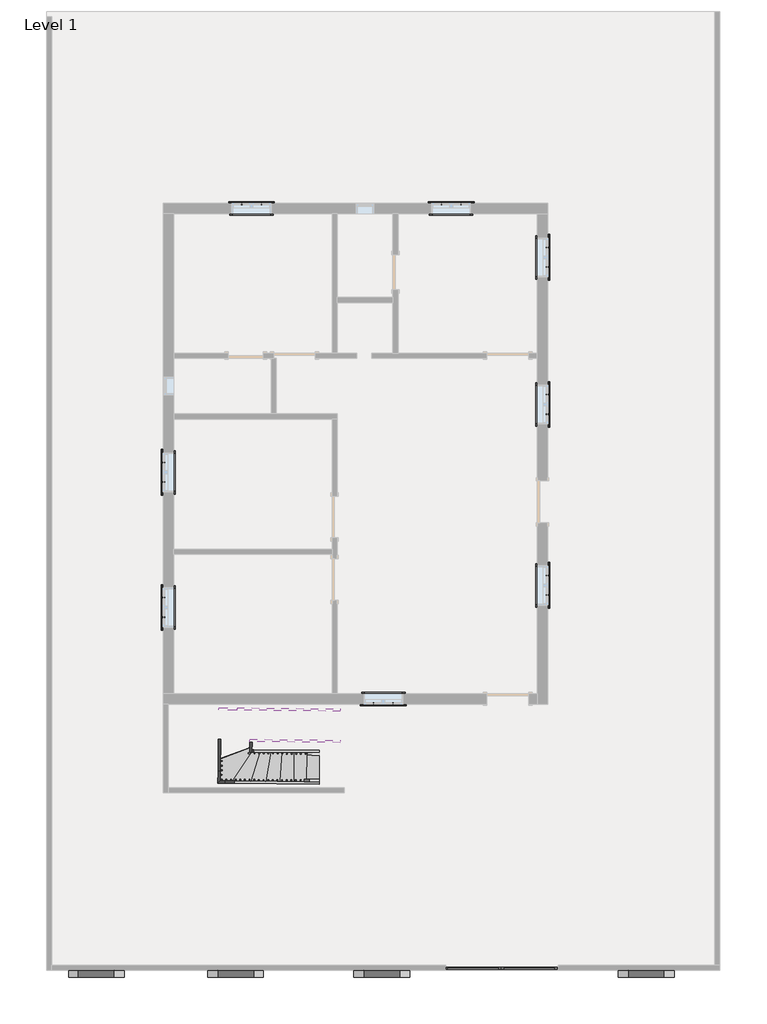
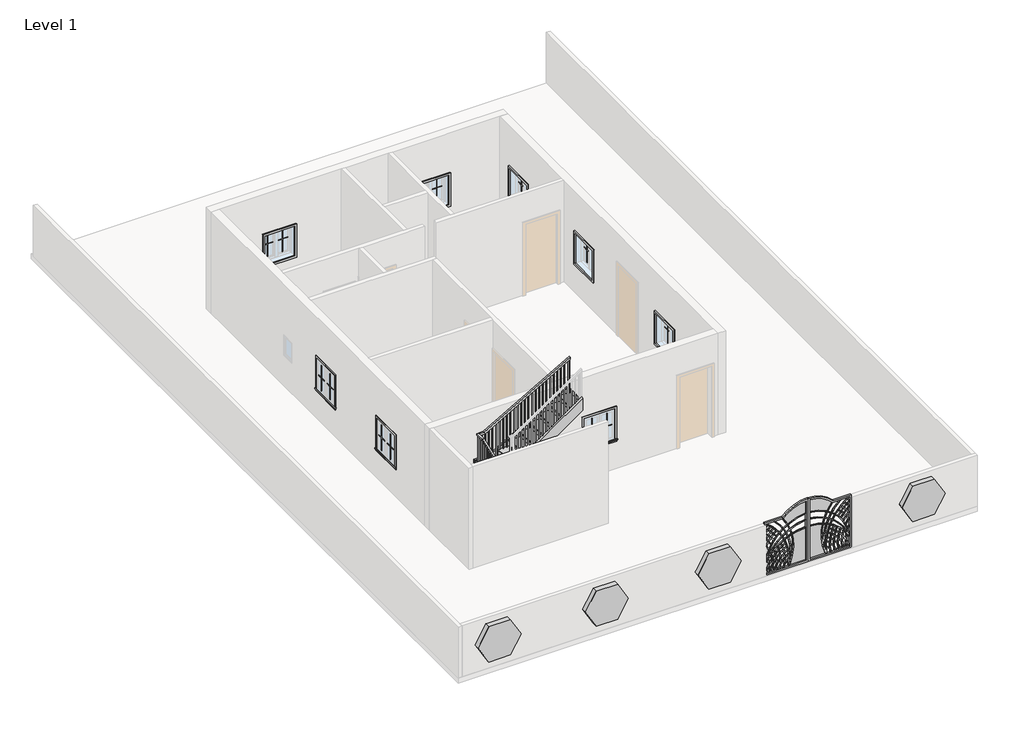
# One storey, part 2 of 2: 34 proxies, 9 members, 1 railing, 1 stair flight.
"""IFC4 building model written with IfcOpenShell, lengths in millimetres."""

from ifc_helpers import new_model, si_unit, frame, origin, place, context, project, spatial, polyline, outline, extrude, faceted_brep, transform, mapped, element, save
from components import generic_models_6bc30956, generic_models_1_generic_models_1_46fdab30, muntin_pattern_2x2_muntin_pattern_2x2_b3fe6957, muntin_pattern_2x2_muntin_pattern_2x2_3e0ecaf2, trim_window_exterior_flat_with_sill_41619996, trim_window_interior_flat_picture_frame_51c85655, stair_flight_bcee568d

model = new_model("IFC4")

# Units and contexts
model_context = context("Model", 3, world=origin())
ifc_project = project(units=[si_unit("LENGTHUNIT", "METRE", prefix="MILLI")], contexts=[model_context])

# Site, building, storey
site = spatial("IfcSite", under=ifc_project)
building = spatial("IfcBuilding", under=site)
storey = spatial("IfcBuildingStorey", under=building, Name="Level 1", Elevation=0.0)

# Proxies
placement = place(None, origin())
generic_models_shape = generic_models_6bc30956(model_context)
element("IfcBuildingElementProxy", 1, Name="Generic Models", at=placement, inside=storey, context=model_context, shape_type="MappedRepresentation", body=[
    mapped(generic_models_shape, transform((2009.5752168, -9655.81366, 0.0), x_axis=(1.0, 0.0, 0.0), y_axis=(0.0, 1.0, 0.0), z_axis=(0.0, 0.0, 1.0))),
])
generic_models_1_generic_models_1_shape = generic_models_1_generic_models_1_46fdab30(model_context)
element("IfcBuildingElementProxy", 2, Name="Generic Models 1 : Generic Models 1", ObjectType="Generic Models 1 : Generic Models 1", at=placement, inside=storey, context=model_context, shape_type="MappedRepresentation", body=[
    mapped(generic_models_1_generic_models_1_shape, transform((0.0, 0.0, 0.0), x_axis=(1.0, 0.0, 0.0), y_axis=(0.0, 1.0, 0.0), z_axis=(0.0, 0.0, 1.0))),
])
muntin_pattern_2x2_muntin_pattern_2x2_shape = muntin_pattern_2x2_muntin_pattern_2x2_b3fe6957(model_context)
element("IfcBuildingElementProxy", 3, Name="Muntin Pattern_2x2 : Muntin Pattern_2x2", ObjectType="Muntin Pattern_2x2 : Muntin Pattern_2x2", at=placement, inside=storey, context=model_context, shape_type="MappedRepresentation", body=[
    mapped(muntin_pattern_2x2_muntin_pattern_2x2_shape, transform((-3662.5622832, 7052.6782079, 984.25), x_axis=(1.0, 0.0, 0.0), y_axis=(0.0, 1.0, 0.0), z_axis=(0.0, 0.0, 1.0))),
])
element("IfcBuildingElementProxy", 4, Name="Muntin Pattern_2x2 : Muntin Pattern_2x2", ObjectType="Muntin Pattern_2x2 : Muntin Pattern_2x2", at=placement, inside=storey, context=model_context, shape_type="MappedRepresentation", body=[
    mapped(muntin_pattern_2x2_muntin_pattern_2x2_shape, transform((709.4127168, 7052.6782079, 984.25), x_axis=(1.0, 0.0, 0.0), y_axis=(0.0, 1.0, 0.0), z_axis=(0.0, 0.0, 1.0))),
])
element("IfcBuildingElementProxy", 5, Name="Muntin Pattern_2x2 : Muntin Pattern_2x2", ObjectType="Muntin Pattern_2x2 : Muntin Pattern_2x2", at=placement, inside=storey, context=model_context, shape_type="MappedRepresentation", body=[
    mapped(muntin_pattern_2x2_muntin_pattern_2x2_shape, transform((3028.7502168, 6095.4157079, 984.25), x_axis=(0.0, -1.0, 0.0), y_axis=(1.0, 0.0, 0.0), z_axis=(0.0, 0.0, 1.0))),
])
element("IfcBuildingElementProxy", 6, Name="Muntin Pattern_2x2 : Muntin Pattern_2x2", ObjectType="Muntin Pattern_2x2 : Muntin Pattern_2x2", at=placement, inside=storey, context=model_context, shape_type="MappedRepresentation", body=[
    mapped(muntin_pattern_2x2_muntin_pattern_2x2_shape, transform((3028.7502168, 2875.9657079, 984.25), x_axis=(0.0, -1.0, 0.0), y_axis=(1.0, 0.0, 0.0), z_axis=(0.0, 0.0, 1.0))),
])
element("IfcBuildingElementProxy", 7, Name="Muntin Pattern_2x2 : Muntin Pattern_2x2", ObjectType="Muntin Pattern_2x2 : Muntin Pattern_2x2", at=placement, inside=storey, context=model_context, shape_type="MappedRepresentation", body=[
    mapped(muntin_pattern_2x2_muntin_pattern_2x2_shape, transform((3028.7502168, -1086.4342921, 984.25), x_axis=(0.0, -1.0, 0.0), y_axis=(1.0, 0.0, 0.0), z_axis=(0.0, 0.0, 1.0))),
])
element("IfcBuildingElementProxy", 8, Name="Muntin Pattern_2x2 : Muntin Pattern_2x2", ObjectType="Muntin Pattern_2x2 : Muntin Pattern_2x2", at=placement, inside=storey, context=model_context, shape_type="MappedRepresentation", body=[
    mapped(muntin_pattern_2x2_muntin_pattern_2x2_shape, transform((-5372.2997832, 961.4407079, 984.25), x_axis=(0.0, 1.0, 0.0), y_axis=(-1.0, 0.0, 0.0), z_axis=(0.0, 0.0, 1.0))),
])
element("IfcBuildingElementProxy", 9, Name="Muntin Pattern_2x2 : Muntin Pattern_2x2", ObjectType="Muntin Pattern_2x2 : Muntin Pattern_2x2", at=placement, inside=storey, context=model_context, shape_type="MappedRepresentation", body=[
    mapped(muntin_pattern_2x2_muntin_pattern_2x2_shape, transform((-5372.2997832, -1997.6592921, 984.25), x_axis=(0.0, 1.0, 0.0), y_axis=(-1.0, 0.0, 0.0), z_axis=(0.0, 0.0, 1.0))),
])
element("IfcBuildingElementProxy", 10, Name="Muntin Pattern_2x2 : Muntin Pattern_2x2", ObjectType="Muntin Pattern_2x2 : Muntin Pattern_2x2", at=placement, inside=storey, context=model_context, shape_type="MappedRepresentation", body=[
    mapped(muntin_pattern_2x2_muntin_pattern_2x2_shape, transform((-347.8622832, -3888.3717921, 984.25), x_axis=(-1.0, 0.0, 0.0), y_axis=(0.0, -1.0, 0.0), z_axis=(0.0, 0.0, 1.0))),
])
muntin_pattern_2x2_muntin_pattern_2x2_2_shape = muntin_pattern_2x2_muntin_pattern_2x2_3e0ecaf2(model_context)
element("IfcBuildingElementProxy", 11, Name="Muntin Pattern_2x2 : Muntin Pattern_2x2", ObjectType="Muntin Pattern_2x2 : Muntin Pattern_2x2", at=placement, inside=storey, context=model_context, shape_type="MappedRepresentation", body=[
    mapped(muntin_pattern_2x2_muntin_pattern_2x2_2_shape, transform((-3233.9372832, 7052.6782079, 984.25), x_axis=(-1.0, 0.0, 0.0), y_axis=(0.0, -1.0, 0.0), z_axis=(0.0, 0.0, 1.0))),
])
element("IfcBuildingElementProxy", 12, Name="Muntin Pattern_2x2 : Muntin Pattern_2x2", ObjectType="Muntin Pattern_2x2 : Muntin Pattern_2x2", at=placement, inside=storey, context=model_context, shape_type="MappedRepresentation", body=[
    mapped(muntin_pattern_2x2_muntin_pattern_2x2_2_shape, transform((1138.0377168, 7052.6782079, 984.25), x_axis=(-1.0, 0.0, 0.0), y_axis=(0.0, -1.0, 0.0), z_axis=(0.0, 0.0, 1.0))),
])
element("IfcBuildingElementProxy", 13, Name="Muntin Pattern_2x2 : Muntin Pattern_2x2", ObjectType="Muntin Pattern_2x2 : Muntin Pattern_2x2", at=placement, inside=storey, context=model_context, shape_type="MappedRepresentation", body=[
    mapped(muntin_pattern_2x2_muntin_pattern_2x2_2_shape, transform((3028.7502168, 5666.7907079, 984.25), x_axis=(0.0, 1.0, 0.0), y_axis=(-1.0, 0.0, 0.0), z_axis=(0.0, 0.0, 1.0))),
])
element("IfcBuildingElementProxy", 14, Name="Muntin Pattern_2x2 : Muntin Pattern_2x2", ObjectType="Muntin Pattern_2x2 : Muntin Pattern_2x2", at=placement, inside=storey, context=model_context, shape_type="MappedRepresentation", body=[
    mapped(muntin_pattern_2x2_muntin_pattern_2x2_2_shape, transform((3028.7502168, 2447.3407079, 984.25), x_axis=(0.0, 1.0, 0.0), y_axis=(-1.0, 0.0, 0.0), z_axis=(0.0, 0.0, 1.0))),
])
element("IfcBuildingElementProxy", 15, Name="Muntin Pattern_2x2 : Muntin Pattern_2x2", ObjectType="Muntin Pattern_2x2 : Muntin Pattern_2x2", at=placement, inside=storey, context=model_context, shape_type="MappedRepresentation", body=[
    mapped(muntin_pattern_2x2_muntin_pattern_2x2_2_shape, transform((3028.7502168, -1515.0592921, 984.25), x_axis=(0.0, 1.0, 0.0), y_axis=(-1.0, 0.0, 0.0), z_axis=(0.0, 0.0, 1.0))),
])
element("IfcBuildingElementProxy", 16, Name="Muntin Pattern_2x2 : Muntin Pattern_2x2", ObjectType="Muntin Pattern_2x2 : Muntin Pattern_2x2", at=placement, inside=storey, context=model_context, shape_type="MappedRepresentation", body=[
    mapped(muntin_pattern_2x2_muntin_pattern_2x2_2_shape, transform((-5372.2997832, 1390.0657079, 984.25), x_axis=(0.0, -1.0, 0.0), y_axis=(1.0, 0.0, 0.0), z_axis=(0.0, 0.0, 1.0))),
])
element("IfcBuildingElementProxy", 17, Name="Muntin Pattern_2x2 : Muntin Pattern_2x2", ObjectType="Muntin Pattern_2x2 : Muntin Pattern_2x2", at=placement, inside=storey, context=model_context, shape_type="MappedRepresentation", body=[
    mapped(muntin_pattern_2x2_muntin_pattern_2x2_2_shape, transform((-5372.2997832, -1569.0342921, 984.25), x_axis=(0.0, -1.0, 0.0), y_axis=(1.0, 0.0, 0.0), z_axis=(0.0, 0.0, 1.0))),
])
element("IfcBuildingElementProxy", 18, Name="Muntin Pattern_2x2 : Muntin Pattern_2x2", ObjectType="Muntin Pattern_2x2 : Muntin Pattern_2x2", at=placement, inside=storey, context=model_context, shape_type="MappedRepresentation", body=[
    mapped(muntin_pattern_2x2_muntin_pattern_2x2_2_shape, transform((-776.4872832, -3888.3717921, 984.25), x_axis=(1.0, 0.0, 0.0), y_axis=(0.0, 1.0, 0.0), z_axis=(0.0, 0.0, 1.0))),
])
trim_window_exterior_flat_with_sill_shape = trim_window_exterior_flat_with_sill_41619996(model_context)
element("IfcBuildingElementProxy", 19, Name="Trim-Window-Exterior-Flat : with Sill", ObjectType="Trim-Window-Exterior-Flat : with Sill", at=placement, inside=storey, context=model_context, shape_type="MappedRepresentation", body=[
    mapped(trim_window_exterior_flat_with_sill_shape, transform((-3448.2497832, 7062.2032079, 1828.8), x_axis=(-1.0, 0.0, 0.0), y_axis=(0.0, 0.0, 1.0), z_axis=(0.0, 1.0, 0.0))),
])
element("IfcBuildingElementProxy", 20, Name="Trim-Window-Exterior-Flat : with Sill", ObjectType="Trim-Window-Exterior-Flat : with Sill", at=placement, inside=storey, context=model_context, shape_type="MappedRepresentation", body=[
    mapped(trim_window_exterior_flat_with_sill_shape, transform((923.7252168, 7062.2032079, 1828.8), x_axis=(-1.0, 0.0, 0.0), y_axis=(0.0, 0.0, 1.0), z_axis=(0.0, 1.0, 0.0))),
])
element("IfcBuildingElementProxy", 21, Name="Trim-Window-Exterior-Flat : with Sill", ObjectType="Trim-Window-Exterior-Flat : with Sill", at=placement, inside=storey, context=model_context, shape_type="MappedRepresentation", body=[
    mapped(trim_window_exterior_flat_with_sill_shape, transform((3038.2752168, 5881.1032079, 1828.8), x_axis=(0.0, 1.0, 0.0), y_axis=(0.0, 0.0, 1.0), z_axis=(1.0, 0.0, 0.0))),
])
element("IfcBuildingElementProxy", 22, Name="Trim-Window-Exterior-Flat : with Sill", ObjectType="Trim-Window-Exterior-Flat : with Sill", at=placement, inside=storey, context=model_context, shape_type="MappedRepresentation", body=[
    mapped(trim_window_exterior_flat_with_sill_shape, transform((3038.2752168, 2661.6532079, 1828.8), x_axis=(0.0, 1.0, 0.0), y_axis=(0.0, 0.0, 1.0), z_axis=(1.0, 0.0, 0.0))),
])
element("IfcBuildingElementProxy", 23, Name="Trim-Window-Exterior-Flat : with Sill", ObjectType="Trim-Window-Exterior-Flat : with Sill", at=placement, inside=storey, context=model_context, shape_type="MappedRepresentation", body=[
    mapped(trim_window_exterior_flat_with_sill_shape, transform((3038.2752168, -1300.7467921, 1828.8), x_axis=(0.0, 1.0, 0.0), y_axis=(0.0, 0.0, 1.0), z_axis=(1.0, 0.0, 0.0))),
])
element("IfcBuildingElementProxy", 24, Name="Trim-Window-Exterior-Flat : with Sill", ObjectType="Trim-Window-Exterior-Flat : with Sill", at=placement, inside=storey, context=model_context, shape_type="MappedRepresentation", body=[
    mapped(trim_window_exterior_flat_with_sill_shape, transform((-5381.8247832, 1175.7532079, 1828.8), x_axis=(0.0, -1.0, 0.0), y_axis=(0.0, 0.0, 1.0), z_axis=(-1.0, 0.0, 0.0))),
])
element("IfcBuildingElementProxy", 25, Name="Trim-Window-Exterior-Flat : with Sill", ObjectType="Trim-Window-Exterior-Flat : with Sill", at=placement, inside=storey, context=model_context, shape_type="MappedRepresentation", body=[
    mapped(trim_window_exterior_flat_with_sill_shape, transform((-5381.8247832, -1783.3467921, 1828.8), x_axis=(0.0, -1.0, 0.0), y_axis=(0.0, 0.0, 1.0), z_axis=(-1.0, 0.0, 0.0))),
])
element("IfcBuildingElementProxy", 26, Name="Trim-Window-Exterior-Flat : with Sill", ObjectType="Trim-Window-Exterior-Flat : with Sill", at=placement, inside=storey, context=model_context, shape_type="MappedRepresentation", body=[
    mapped(trim_window_exterior_flat_with_sill_shape, transform((-562.1747832, -3897.8967921, 1828.8), x_axis=(1.0, 0.0, 0.0), y_axis=(0.0, 0.0, 1.0), z_axis=(0.0, -1.0, 0.0))),
])
trim_window_interior_flat_picture_frame_shape = trim_window_interior_flat_picture_frame_51c85655(model_context)
element("IfcBuildingElementProxy", 27, Name="Trim-Window-Interior-Flat : Picture Frame", ObjectType="Trim-Window-Interior-Flat : Picture Frame", at=placement, inside=storey, context=model_context, shape_type="MappedRepresentation", body=[
    mapped(trim_window_interior_flat_picture_frame_shape, transform((-3448.2497832, 6833.6032079, 1828.8), x_axis=(1.0, 0.0, 0.0), y_axis=(0.0, 0.0, 1.0), z_axis=(0.0, -1.0, 0.0))),
])
element("IfcBuildingElementProxy", 28, Name="Trim-Window-Interior-Flat : Picture Frame", ObjectType="Trim-Window-Interior-Flat : Picture Frame", at=placement, inside=storey, context=model_context, shape_type="MappedRepresentation", body=[
    mapped(trim_window_interior_flat_picture_frame_shape, transform((923.7252168, 6833.6032079, 1828.8), x_axis=(1.0, 0.0, 0.0), y_axis=(0.0, 0.0, 1.0), z_axis=(0.0, -1.0, 0.0))),
])
element("IfcBuildingElementProxy", 29, Name="Trim-Window-Interior-Flat : Picture Frame", ObjectType="Trim-Window-Interior-Flat : Picture Frame", at=placement, inside=storey, context=model_context, shape_type="MappedRepresentation", body=[
    mapped(trim_window_interior_flat_picture_frame_shape, transform((2809.6752168, 5881.1032079, 1828.8), x_axis=(0.0, -1.0, 0.0), y_axis=(0.0, 0.0, 1.0), z_axis=(-1.0, 0.0, 0.0))),
])
element("IfcBuildingElementProxy", 30, Name="Trim-Window-Interior-Flat : Picture Frame", ObjectType="Trim-Window-Interior-Flat : Picture Frame", at=placement, inside=storey, context=model_context, shape_type="MappedRepresentation", body=[
    mapped(trim_window_interior_flat_picture_frame_shape, transform((2809.6752168, 2661.6532079, 1828.8), x_axis=(0.0, -1.0, 0.0), y_axis=(0.0, 0.0, 1.0), z_axis=(-1.0, 0.0, 0.0))),
])
element("IfcBuildingElementProxy", 31, Name="Trim-Window-Interior-Flat : Picture Frame", ObjectType="Trim-Window-Interior-Flat : Picture Frame", at=placement, inside=storey, context=model_context, shape_type="MappedRepresentation", body=[
    mapped(trim_window_interior_flat_picture_frame_shape, transform((2809.6752168, -1300.7467921, 1828.8), x_axis=(0.0, -1.0, 0.0), y_axis=(0.0, 0.0, 1.0), z_axis=(-1.0, 0.0, 0.0))),
])
element("IfcBuildingElementProxy", 32, Name="Trim-Window-Interior-Flat : Picture Frame", ObjectType="Trim-Window-Interior-Flat : Picture Frame", at=placement, inside=storey, context=model_context, shape_type="MappedRepresentation", body=[
    mapped(trim_window_interior_flat_picture_frame_shape, transform((-5153.2247832, 1175.7532079, 1828.8), x_axis=(0.0, 1.0, 0.0), y_axis=(0.0, 0.0, 1.0), z_axis=(1.0, 0.0, 0.0))),
])
element("IfcBuildingElementProxy", 33, Name="Trim-Window-Interior-Flat : Picture Frame", ObjectType="Trim-Window-Interior-Flat : Picture Frame", at=placement, inside=storey, context=model_context, shape_type="MappedRepresentation", body=[
    mapped(trim_window_interior_flat_picture_frame_shape, transform((-5153.2247832, -1783.3467921, 1828.8), x_axis=(0.0, 1.0, 0.0), y_axis=(0.0, 0.0, 1.0), z_axis=(1.0, 0.0, 0.0))),
])
element("IfcBuildingElementProxy", 34, Name="Trim-Window-Interior-Flat : Picture Frame", ObjectType="Trim-Window-Interior-Flat : Picture Frame", at=placement, inside=storey, context=model_context, shape_type="MappedRepresentation", body=[
    mapped(trim_window_interior_flat_picture_frame_shape, transform((-562.1747832, -3669.2967921, 1828.8), x_axis=(-1.0, 0.0, 0.0), y_axis=(0.0, 0.0, 1.0), z_axis=(0.0, 1.0, 0.0))),
])

# Members
element("IfcMember", 35, ObjectType="Stringer - 2\" Width", at=placement, inside=storey, context=model_context, shape_type="SweptSolid", body=[
    extrude(outline(polyline([(-105.6395382, -202.4353776), (0.0, 0.0), (2328.2458671, 0.0), (2169.1880402, -304.8), (90.52017, -304.8), (-105.6395382, -202.4353776)])), frame((-1968.9977307, -5651.1672049, 228.3413982), z_axis=(0.010736031619565219, 0.9999423671517593, 0.0), x_axis=(-0.8864958884204133, 0.009517996437940355, 0.4626385711951713)), (0.0, 0.0, 1.0), 50.8),
])
element("IfcMember", 36, ObjectType="Stringer - 2\" Width", at=placement, inside=storey, context=model_context, shape_type="SweptSolid", body=[
    extrude(outline(polyline([(-4032.4327287, -5578.2098967), (-4032.9781191, -5629.006969), (-4182.4018504, -5627.4026586), (-4131.0593878, -5577.1509768), (-4032.4327287, -5578.2098967)])), frame((0.0, 0.0, 961.6719334), z_axis=(0.0, 0.0, 1.0), x_axis=(1.0, 0.0, 0.0)), (0.0, 0.0, 1.0), 343.8058061),
])
element("IfcMember", 37, ObjectType="Stringer - 2\" Width", at=placement, inside=storey, context=model_context, shape_type="SweptSolid", body=[
    extrude(outline(polyline([(-4131.0593878, -5577.1509768), (-4182.4018504, -5627.4026586), (-4179.6442274, -5370.5606366), (-4128.8471552, -5371.106027), (-4131.0593878, -5577.1509768)])), frame((0.0, 0.0, 961.6719334), z_axis=(0.0, 0.0, 1.0), x_axis=(1.0, 0.0, 0.0)), (0.0, 0.0, 1.0), 343.8058061),
])
element("IfcMember", 38, ObjectType="Stringer - 2\" Width", at=placement, inside=storey, context=model_context, shape_type="SweptSolid", body=[
    extrude(outline(polyline([(110.9788635, -325.4014815), (0.0, 0.0), (1419.3210826, 0.0), (1526.5904374, -314.5248191), (1494.6989405, -325.4014816), (110.9788635, -325.4014815)])), frame((-4128.8471552, -5371.106027, 961.6719334), z_axis=(-0.9999423671517594, 0.010736031619565323, 0.0), x_axis=(0.01016131936269789, 0.9464142894665318, 0.3227951986668468)), (0.0, 0.0, 1.0), 50.8),
])
element("IfcMember", 39, ObjectType="Stringer - 2\" Width", at=placement, inside=storey, context=model_context, shape_type="SweptSolid", body=[
    extrude(outline(polyline([(-4165.2220526, -4027.2948827), (-4164.6766622, -3976.4978105), (-3763.6581151, -3980.8034064), (-3764.2035055, -4031.6004787), (-4165.2220526, -4027.2948827)])), frame((0.0, 0.0, 1430.0968076), z_axis=(0.0, 0.0, 1.0), x_axis=(1.0, 0.0, 0.0)), (0.0, 0.0, 1.0), 322.0391291),
])
element("IfcMember", 40, ObjectType="Stringer - 2\" Width", at=placement, inside=storey, context=model_context, shape_type="SweptSolid", body=[
    extrude(outline(polyline([(-111.9640108, -160.4153284), (0.0, 0.0), (1801.1015507, 0.0), (1588.362339, -304.8), (94.9016984, -304.8), (-111.9640108, -160.4153284)])), frame((-1961.6349602, -4965.4067295, 195.6246848), z_axis=(0.010736031619565368, 0.9999423671517593, 0.0), x_axis=(-0.8199685195580251, 0.008803715336213087, 0.5723409137307062)), (0.0, 0.0, 1.0), 50.8),
])
element("IfcMember", 41, ObjectType="Stringer - 2\" Width", at=placement, inside=storey, context=model_context, shape_type="SweptSolid", body=[
    extrude(outline(polyline([(451.3522078, -304.8), (7.554265, -5.1014262), (10.999279, 0.0), (408.4725128, 0.0), (831.8908901, -285.9361695), (819.1520678, -304.8), (451.3522078, -304.8)])), frame((-3438.4815323, -4949.5503441, 881.1097108), z_axis=(-0.9999423671517593, 0.0107360316195659, 0.0), x_axis=(0.006008376943933793, 0.5596137266499716, 0.8287317879455516)), (0.0, 0.0, 1.0), 50.8),
])
element("IfcMember", 42, ObjectType="Stringer - 2\" Width", at=placement, inside=storey, context=model_context, shape_type="SweptSolid", body=[
    extrude(outline(polyline([(215.732707, -304.8), (0.0, 0.0), (2421.4097535, 0.0), (2637.1424605, -304.8), (215.732707, -304.8)])), frame((-3486.8243477, -4720.4181286, 1357.1256311), z_axis=(0.010736031619565212, 0.9999423671517593, 0.0), x_axis=(0.8161886957592972, -0.008763132689499912, 0.5777189804915567)), (0.0, 0.0, 1.0), 50.8),
])
element("IfcMember", 43, ObjectType="Stringer - 2\" Width", at=placement, inside=storey, context=model_context, shape_type="SweptSolid", body=[
    extrude(outline(polyline([(161.6856691, -278.5084291), (0.0, 0.0), (2614.6236412, 0.0), (2776.3093103, -278.508429), (161.6856691, -278.5084291)])), frame((-3764.2035055, -4031.6004787, 1430.0968076), z_axis=(0.010736031619565321, 0.9999423671517593, 0.0), x_axis=(0.8647780740833304, -0.009284819857879248, 0.5020683964410951)), (0.0, 0.0, 1.0), 50.8),
])

# Railing
element("IfcRailing", 44, ObjectType="Handrail - Rectangular", at=placement, inside=storey, context=model_context, shape_type="SolidModel", body=[
    faceted_brep([(-1968.4523403, -5600.3701326, 1083.7333333), (-1968.4523403, -5600.3701326, 1026.1388957), (-1967.9069499, -5549.5730604, 1026.1388957), (-1967.9069499, -5549.5730604, 1083.7333333), (-4009.5042766, -5578.4560715, 2174.1579081), (-4022.2220752, -5578.319525, 2123.3579081), (-4021.6766848, -5527.5224527, 2123.3579081), (-4008.9588862, -5527.6589993, 2174.1579081), (-4131.0593878, -5577.1509768, 2174.1579081), (-4131.0593878, -5577.1509768, 2123.3579081), (-4079.7169251, -5526.8992949, 2123.3579081), (-4079.7169251, -5526.8992949, 2174.1579081), (-4129.1695675, -5401.1351667, 2174.1579081), (-4129.079122, -5392.7111679, 2123.3579081), (-4078.2820498, -5393.2565584, 2123.3579081), (-4078.3724953, -5401.6805571, 2174.1579081), (-4117.5603361, -4319.8639155, 2542.9490097), (-4117.4698906, -4311.4399167, 2492.1490097), (-4066.6728183, -4311.9853071, 2492.1490097), (-4066.7632639, -4320.4093059, 2542.9490097), (-4114.4249804, -4027.8402731, 2542.9490097), (-4114.4249804, -4027.8402731, 2492.1490097), (-4064.1732985, -4079.1827358, 2492.1490097), (-4064.1732985, -4079.1827358, 2542.9490097), (-3933.3337165, -4029.7845867, 2542.9490097), (-3919.5861077, -4029.93219, 2492.1490097), (-3920.1314981, -4080.7292622, 2492.1490097), (-3933.8791069, -4080.581659, 2542.9490097), (-1503.1343086, -4055.8767882, 3962.4), (-1503.679699, -4106.6738604, 3962.4), (-1503.679699, -4106.6738604, 3903.5701828), (-1503.1343086, -4055.8767882, 3903.5701828)], [[[0, 1, 2, 3]], [[1, 0, 4, 5]], [[2, 1, 5, 6]], [[3, 2, 6, 7]], [[0, 3, 7, 4]], [[5, 4, 8, 9]], [[6, 5, 9, 10]], [[7, 6, 10, 11]], [[4, 7, 11, 8]], [[9, 8, 12, 13]], [[10, 9, 13, 14]], [[11, 10, 14, 15]], [[8, 11, 15, 12]], [[13, 12, 16, 17]], [[14, 13, 17, 18]], [[15, 14, 18, 19]], [[12, 15, 19, 16]], [[17, 16, 20, 21]], [[18, 17, 21, 22]], [[19, 18, 22, 23]], [[16, 19, 23, 20]], [[21, 20, 24, 25]], [[22, 21, 25, 26]], [[23, 22, 26, 27]], [[20, 23, 27, 24]], [[28, 29, 30, 31]], [[25, 24, 28, 31]], [[26, 25, 31, 30]], [[27, 26, 30, 29]], [[24, 27, 29, 28]]]),
    extrude(outline(polyline([(234.1631202, 19.05), (1226.6129544, 19.05), (1226.6129544, 0.0), (223.0368797, 0.0), (234.1631202, 19.05)])), frame((-1540.0233365, -4090.4077365, 4105.2796211), z_axis=(0.010736031619565153, 0.9999423671517594, 0.0), x_axis=(0.0, 0.0, -1.0)), (0.0, 0.0, 1.0), 19.05),
    extrude(outline(polyline([(234.1631202, 19.05), (1167.2730054, 19.05), (1167.2730054, 0.0), (223.0368798, 0.0), (234.1631202, 19.05)])), frame((-1641.617481, -4089.3169557, 4045.9396721), z_axis=(0.010736031619565153, 0.9999423671517594, 0.0), x_axis=(0.0, 0.0, -1.0)), (0.0, 0.0, 1.0), 19.05),
    extrude(outline(polyline([(234.1631202, 19.05), (1107.9330563, 19.05), (1107.9330563, 0.0), (223.0368797, 0.0), (234.1631202, 19.05)])), frame((-1743.2116255, -4088.2261749, 3986.599723), z_axis=(0.010736031619565153, 0.9999423671517594, 0.0), x_axis=(0.0, 0.0, -1.0)), (0.0, 0.0, 1.0), 19.05),
    extrude(outline(polyline([(234.1631202, 19.05), (1217.9264407, 19.05), (1217.9264407, 0.0), (223.0368798, 0.0), (234.1631202, 19.05)])), frame((-1844.80577, -4087.1353941, 3927.259774), z_axis=(0.010736031619565153, 0.9999423671517594, 0.0), x_axis=(0.0, 0.0, -1.0)), (0.0, 0.0, 1.0), 19.05),
    extrude(outline(polyline([(234.1631203, 19.05), (1158.5864917, 19.05), (1158.5864917, 0.0), (223.0368798, 0.0), (234.1631203, 19.05)])), frame((-1946.3999145, -4086.0446133, 3867.919825), z_axis=(0.010736031619565153, 0.9999423671517594, 0.0), x_axis=(0.0, 0.0, -1.0)), (0.0, 0.0, 1.0), 19.05),
    extrude(outline(polyline([(234.1631202, 19.05), (1099.2465426, 19.05), (1099.2465426, 0.0), (223.0368798, 0.0), (234.1631202, 19.05)])), frame((-2047.994059, -4084.9538324, 3808.5798759), z_axis=(0.010736031619565153, 0.9999423671517594, 0.0), x_axis=(0.0, 0.0, -1.0)), (0.0, 0.0, 1.0), 19.05),
    extrude(outline(polyline([(234.1631202, 19.0499999), (1209.2399269, 19.0499999), (1209.2399269, 0.0), (223.0368798, 0.0), (234.1631202, 19.0499999)])), frame((-2149.5882036, -4083.8630516, 3749.2399269), z_axis=(0.010736031619565153, 0.9999423671517594, 0.0), x_axis=(0.0, 0.0, -1.0)), (0.0, 0.0, 1.0), 19.05),
    extrude(outline(polyline([(234.1631202, 19.0499999), (1149.8999778, 19.0499999), (1149.8999778, 0.0), (223.0368797, 0.0), (234.1631202, 19.0499999)])), frame((-2251.1823481, -4082.7722708, 3689.8999778), z_axis=(0.010736031619565153, 0.9999423671517594, 0.0), x_axis=(0.0, 0.0, -1.0)), (0.0, 0.0, 1.0), 19.05),
    extrude(outline(polyline([(234.1631202, 19.05), (1259.8933621, 19.05), (1259.8933621, 0.0), (223.0368798, 0.0), (234.1631202, 19.05)])), frame((-2352.7764926, -4081.68149, 3630.5600288), z_axis=(0.010736031619565153, 0.9999423671517594, 0.0), x_axis=(0.0, 0.0, -1.0)), (0.0, 0.0, 1.0), 19.05),
    extrude(outline(polyline([(234.1631203, 19.05), (1200.5534131, 19.05), (1200.5534131, 0.0), (223.0368798, 0.0), (234.1631203, 19.05)])), frame((-2454.3706371, -4080.5907092, 3571.2200798), z_axis=(0.010736031619565153, 0.9999423671517594, 0.0), x_axis=(0.0, 0.0, -1.0)), (0.0, 0.0, 1.0), 19.05),
    extrude(outline(polyline([(234.1631202, 19.05), (1141.213464, 19.05), (1141.213464, 0.0), (223.0368798, 0.0), (234.1631202, 19.05)])), frame((-2555.9647816, -4079.4999284, 3511.8801307), z_axis=(0.010736031619565153, 0.9999423671517594, 0.0), x_axis=(0.0, 0.0, -1.0)), (0.0, 0.0, 1.0), 19.05),
    extrude(outline(polyline([(234.1631203, 19.05), (1251.2068484, 19.05), (1251.2068484, 0.0), (223.0368798, 0.0), (234.1631203, 19.05)])), frame((-2657.5589261, -4078.4091476, 3452.5401817), z_axis=(0.010736031619565153, 0.9999423671517594, 0.0), x_axis=(0.0, 0.0, -1.0)), (0.0, 0.0, 1.0), 19.05),
    extrude(outline(polyline([(234.1631202, 19.05), (1191.8668993, 19.05), (1191.8668993, 0.0), (223.0368797, 0.0), (234.1631202, 19.05)])), frame((-2759.1530706, -4077.3183668, 3393.2002326), z_axis=(0.010736031619565153, 0.9999423671517594, 0.0), x_axis=(0.0, 0.0, -1.0)), (0.0, 0.0, 1.0), 19.05),
    extrude(outline(polyline([(234.1631202, 19.05), (1132.5269503, 19.05), (1132.5269503, 0.0), (223.0368798, 0.0), (234.1631202, 19.05)])), frame((-2860.7472151, -4076.2275859, 3333.8602836), z_axis=(0.010736031619565153, 0.9999423671517594, 0.0), x_axis=(0.0, 0.0, -1.0)), (0.0, 0.0, 1.0), 19.05),
    extrude(outline(polyline([(234.1631202, 19.05), (1242.5203345, 19.05), (1242.5203345, 0.0), (223.0368797, 0.0), (234.1631202, 19.05)])), frame((-2962.3413596, -4075.1368051, 3274.5203345), z_axis=(0.010736031619565153, 0.9999423671517594, 0.0), x_axis=(0.0, 0.0, -1.0)), (0.0, 0.0, 1.0), 19.05),
    extrude(outline(polyline([(234.1631202, 19.05), (1183.1803855, 19.05), (1183.1803855, 0.0), (223.0368798, 0.0), (234.1631202, 19.05)])), frame((-3063.9355041, -4074.0460243, 3215.1803855), z_axis=(0.010736031619565153, 0.9999423671517594, 0.0), x_axis=(0.0, 0.0, -1.0)), (0.0, 0.0, 1.0), 19.05),
    extrude(outline(polyline([(234.1631203, 19.05), (1123.8404365, 19.05), (1123.8404365, 0.0), (223.0368798, 0.0), (234.1631203, 19.05)])), frame((-3165.5296486, -4072.9552435, 3155.8404365), z_axis=(0.010736031619565153, 0.9999423671517594, 0.0), x_axis=(0.0, 0.0, -1.0)), (0.0, 0.0, 1.0), 19.05),
    extrude(outline(polyline([(234.1631202, 19.05), (1233.8338207, 19.05), (1233.8338207, 0.0), (223.0368798, 0.0), (234.1631202, 19.05)])), frame((-3267.1237931, -4071.8644627, 3096.5004874), z_axis=(0.010736031619565153, 0.9999423671517594, 0.0), x_axis=(0.0, 0.0, -1.0)), (0.0, 0.0, 1.0), 19.05),
    extrude(outline(polyline([(234.1631202, 19.05), (1174.4938717, 19.05), (1174.4938717, 0.0), (223.0368798, 0.0), (234.1631202, 19.05)])), frame((-3368.7179376, -4070.7736819, 3037.1605384), z_axis=(0.010736031619565153, 0.9999423671517594, 0.0), x_axis=(0.0, 0.0, -1.0)), (0.0, 0.0, 1.0), 19.05),
    extrude(outline(polyline([(234.1631202, 19.05), (1115.1539226, 19.05), (1115.1539226, 0.0), (223.0368797, 0.0), (234.1631202, 19.05)])), frame((-3470.3120821, -4069.6829011, 2977.8205893), z_axis=(0.010736031619565153, 0.9999423671517594, 0.0), x_axis=(0.0, 0.0, -1.0)), (0.0, 0.0, 1.0), 19.05),
    extrude(outline(polyline([(234.1631202, 19.05), (1225.147307, 19.05), (1225.147307, 0.0), (223.0368798, 0.0), (234.1631202, 19.05)])), frame((-3571.9062266, -4068.5921203, 2918.4806403), z_axis=(0.010736031619565153, 0.9999423671517594, 0.0), x_axis=(0.0, 0.0, -1.0)), (0.0, 0.0, 1.0), 19.05),
    extrude(outline(polyline([(234.1631203, 19.05), (1165.807358, 19.05), (1165.807358, 0.0), (223.0368798, 0.0), (234.1631203, 19.05)])), frame((-3673.5003711, -4067.5013394, 2859.1406913), z_axis=(0.010736031619565153, 0.9999423671517594, 0.0), x_axis=(0.0, 0.0, -1.0)), (0.0, 0.0, 1.0), 19.05),
    extrude(outline(polyline([(234.1631202, 19.05), (1106.4674089, 19.05), (1106.4674089, 0.0), (223.0368798, 0.0), (234.1631202, 19.05)])), frame((-3775.0945156, -4066.4105586, 2799.8007422), z_axis=(0.010736031619565153, 0.9999423671517594, 0.0), x_axis=(0.0, 0.0, -1.0)), (0.0, 0.0, 1.0), 19.05),
    extrude(outline(polyline([(234.1631203, 19.05), (1047.1274599, 19.05), (1047.1274599, 0.0), (223.0368798, 0.0), (234.1631203, 19.05)])), frame((-3876.6886601, -4065.3197778, 2740.4607932), z_axis=(0.010736031619565153, 0.9999423671517594, 0.0), x_axis=(0.0, 0.0, -1.0)), (0.0, 0.0, 1.0), 19.05),
    extrude(outline(polyline([(-3997.1271853, -4044.9755735), (-3978.0782832, -4045.1800949), (-3978.2828046, -4064.228997), (-3997.3317067, -4064.0244756), (-3997.1271853, -4044.9755735)])), frame((0.0, 0.0, 1693.3333333), z_axis=(0.0, 0.0, 1.0), x_axis=(1.0, 0.0, 0.0)), (0.0, 0.0, 1.0), 798.8156763),
    extrude(outline(polyline([(-4099.7439368, -4139.1293032), (-4099.5394154, -4120.0804011), (-4080.4905133, -4120.2849225), (-4080.6950347, -4139.3338246), (-4099.7439368, -4139.1293032)])), frame((0.0, 0.0, 1693.3333333), z_axis=(0.0, 0.0, 1.0), x_axis=(1.0, 0.0, 0.0)), (0.0, 0.0, 1.0), 798.8156763),
    extrude(outline(polyline([(-4100.8347176, -4240.7234477), (-4100.6301962, -4221.6745456), (-4081.5812941, -4221.879067), (-4081.7858155, -4240.9279691), (-4100.8347176, -4240.7234477)])), frame((0.0, 0.0, 1524.0), z_axis=(0.0, 0.0, 1.0), x_axis=(1.0, 0.0, 0.0)), (0.0, 0.0, 1.0), 968.1490097),
    extrude(outline(polyline([(231.8485214, 19.05), (1189.524158, 19.05), (1189.524158, 0.0), (225.3514786, 0.0), (231.8485214, 19.05)])), frame((-4082.6720749, -4323.4732115, 2713.524158), z_axis=(-0.9999423671517593, 0.010736031619565137, 0.0), x_axis=(0.0, 0.0, -1.0)), (0.0, 0.0, 1.0), 19.05),
    extrude(outline(polyline([(231.8485214, 19.05), (1154.8732631, 19.05), (1154.8732631, 0.0), (225.3514786, 0.0), (231.8485214, 19.05)])), frame((-4083.7628557, -4425.067356, 2678.8732631), z_axis=(-0.9999423671517593, 0.010736031619565137, 0.0), x_axis=(0.0, 0.0, -1.0)), (0.0, 0.0, 1.0), 19.05),
    extrude(outline(polyline([(231.8485214, 19.05), (1120.2223682, 19.05), (1120.2223682, 0.0), (225.3514786, 0.0), (231.8485214, 19.05)])), frame((-4084.8536366, -4526.6615005, 2644.2223682), z_axis=(-0.9999423671517593, 0.010736031619565137, 0.0), x_axis=(0.0, 0.0, -1.0)), (0.0, 0.0, 1.0), 19.05),
    extrude(outline(polyline([(231.8485214, 19.05), (1085.5714733, 19.05), (1085.5714733, 0.0), (225.3514786, 0.0), (231.8485214, 19.05)])), frame((-4085.9444174, -4628.255645, 2609.5714733), z_axis=(-0.9999423671517593, 0.010736031619565137, 0.0), x_axis=(0.0, 0.0, -1.0)), (0.0, 0.0, 1.0), 19.05),
    extrude(outline(polyline([(231.8485214, 19.05), (1220.2539118, 19.05), (1220.2539118, 0.0), (225.3514786, 0.0), (231.8485214, 19.05)])), frame((-4087.0351982, -4729.8497895, 2574.9205785), z_axis=(-0.9999423671517593, 0.010736031619565137, 0.0), x_axis=(0.0, 0.0, -1.0)), (0.0, 0.0, 1.0), 19.05),
    extrude(outline(polyline([(231.8485214, 19.05), (1185.6030169, 19.05), (1185.6030169, 0.0), (225.3514786, 0.0), (231.8485214, 19.05)])), frame((-4088.125979, -4831.443934, 2540.2696836), z_axis=(-0.9999423671517593, 0.010736031619565137, 0.0), x_axis=(0.0, 0.0, -1.0)), (0.0, 0.0, 1.0), 19.05),
    extrude(outline(polyline([(231.8485214, 19.05), (1150.952122, 19.05), (1150.952122, 0.0), (225.3514786, 0.0), (231.8485214, 19.05)])), frame((-4089.2167598, -4933.0380785, 2505.6187887), z_axis=(-0.9999423671517593, 0.010736031619565137, 0.0), x_axis=(0.0, 0.0, -1.0)), (0.0, 0.0, 1.0), 19.05),
    extrude(outline(polyline([(231.8485214, 19.05), (1116.3012271, 19.05), (1116.3012271, 0.0), (225.3514786, 0.0), (231.8485214, 19.05)])), frame((-4090.3075406, -5034.632223, 2470.9678938), z_axis=(-0.9999423671517593, 0.010736031619565137, 0.0), x_axis=(0.0, 0.0, -1.0)), (0.0, 0.0, 1.0), 19.05),
    extrude(outline(polyline([(231.8485214, 19.05), (1250.9836656, 19.05), (1250.9836656, 0.0), (225.3514786, 0.0), (231.8485214, 19.05)])), frame((-4091.3983214, -5136.2263675, 2436.3169989), z_axis=(-0.9999423671517593, 0.010736031619565137, 0.0), x_axis=(0.0, 0.0, -1.0)), (0.0, 0.0, 1.0), 19.05),
    extrude(outline(polyline([(231.8485214, 19.05), (1216.3327708, 19.05), (1216.3327708, 0.0), (225.3514786, 0.0), (231.8485214, 19.05)])), frame((-4092.4891022, -5237.820512, 2401.6661041), z_axis=(-0.9999423671517593, 0.010736031619565137, 0.0), x_axis=(0.0, 0.0, -1.0)), (0.0, 0.0, 1.0), 19.05),
    extrude(outline(polyline([(231.8485214, 19.05), (1181.6818759, 19.05), (1181.6818759, 0.0), (225.3514786, 0.0), (231.8485214, 19.05)])), frame((-4093.5798831, -5339.4146565, 2367.0152092), z_axis=(-0.9999423671517593, 0.010736031619565137, 0.0), x_axis=(0.0, 0.0, -1.0)), (0.0, 0.0, 1.0), 19.05),
    extrude(outline(polyline([(-4113.9240874, -5459.8531817), (-4113.719566, -5440.8042796), (-4094.6706639, -5441.008801), (-4094.8751853, -5460.0577031), (-4113.9240874, -5459.8531817)])), frame((0.0, 0.0, 1185.3333333), z_axis=(0.0, 0.0, 1.0), x_axis=(1.0, 0.0, 0.0)), (0.0, 0.0, 1.0), 938.0245748),
    extrude(outline(polyline([(-4092.2344893, -5561.6919112), (-4111.2833914, -5561.4873898), (-4111.07887, -5542.4384877), (-4092.0299679, -5542.6430091), (-4092.2344893, -5561.6919112)])), frame((0.0, 0.0, 1185.3333333), z_axis=(0.0, 0.0, 1.0), x_axis=(1.0, 0.0, 0.0)), (0.0, 0.0, 1.0), 938.0245748),
    extrude(outline(polyline([(223.5115966, 19.05), (1154.9316075, 19.05), (1154.9316075, 0.0), (233.6884033, 0.0), (223.5115966, 19.05)])), frame((-3990.6403448, -5562.782692, 2340.2649408), z_axis=(0.010736031619565252, 0.9999423671517594, 0.0), x_axis=(0.0, 0.0, -1.0)), (0.0, 0.0, 1.0), 19.05),
    extrude(outline(polyline([(223.5115967, 19.05), (1100.6553053, 19.05), (1100.6553053, 0.0), (233.6884034, 0.0), (223.5115967, 19.05)])), frame((-3889.0462003, -5563.8734728, 2285.9886386), z_axis=(0.010736031619565252, 0.9999423671517594, 0.0), x_axis=(0.0, 0.0, -1.0)), (0.0, 0.0, 1.0), 19.05),
    extrude(outline(polyline([(223.5115967, 19.05), (1215.7123363, 19.05), (1215.7123363, 0.0), (233.6884033, 0.0), (223.5115967, 19.05)])), frame((-3787.4520558, -5564.9642536, 2231.7123363), z_axis=(0.010736031619565252, 0.9999423671517594, 0.0), x_axis=(0.0, 0.0, -1.0)), (0.0, 0.0, 1.0), 19.05),
    extrude(outline(polyline([(223.5115967, 19.05), (1161.4360341, 19.05), (1161.4360341, 0.0), (233.6884034, 0.0), (223.5115967, 19.05)])), frame((-3685.8579113, -5566.0550344, 2177.4360341), z_axis=(0.010736031619565252, 0.9999423671517594, 0.0), x_axis=(0.0, 0.0, -1.0)), (0.0, 0.0, 1.0), 19.05),
    extrude(outline(polyline([(223.5115967, 19.05), (1107.1597318, 19.05), (1107.1597318, 0.0), (233.6884033, 0.0), (223.5115967, 19.05)])), frame((-3584.2637668, -5567.1458152, 2123.1597318), z_axis=(0.010736031619565252, 0.9999423671517594, 0.0), x_axis=(0.0, 0.0, -1.0)), (0.0, 0.0, 1.0), 19.05),
    extrude(outline(polyline([(223.5115966, 19.05), (1052.8834295, 19.05), (1052.8834295, 0.0), (233.6884033, 0.0), (223.5115966, 19.05)])), frame((-3482.6696223, -5568.236596, 2068.8834295), z_axis=(0.010736031619565252, 0.9999423671517594, 0.0), x_axis=(0.0, 0.0, -1.0)), (0.0, 0.0, 1.0), 19.05),
    extrude(outline(polyline([(223.5115967, 19.05), (1167.9404606, 19.05), (1167.9404606, 0.0), (233.6884034, 0.0), (223.5115967, 19.05)])), frame((-3381.0754778, -5569.3273769, 2014.6071273), z_axis=(0.010736031619565252, 0.9999423671517594, 0.0), x_axis=(0.0, 0.0, -1.0)), (0.0, 0.0, 1.0), 19.05),
    extrude(outline(polyline([(223.5115966, 19.05), (1113.6641583, 19.05), (1113.6641583, 0.0), (233.6884033, 0.0), (223.5115966, 19.05)])), frame((-3279.4813333, -5570.4181577, 1960.330825), z_axis=(0.010736031619565252, 0.9999423671517594, 0.0), x_axis=(0.0, 0.0, -1.0)), (0.0, 0.0, 1.0), 19.05),
    extrude(outline(polyline([(223.5115967, 19.05), (1059.3878561, 19.05), (1059.3878561, 0.0), (233.6884034, 0.0), (223.5115967, 19.05)])), frame((-3177.8871888, -5571.5089385, 1906.0545228), z_axis=(0.010736031619565252, 0.9999423671517594, 0.0), x_axis=(0.0, 0.0, -1.0)), (0.0, 0.0, 1.0), 19.05),
    extrude(outline(polyline([(223.5115966, 19.05), (1174.4448872, 19.05), (1174.4448872, 0.0), (233.6884033, 0.0), (223.5115966, 19.05)])), frame((-3076.2930443, -5572.5997193, 1851.7782205), z_axis=(0.010736031619565252, 0.9999423671517594, 0.0), x_axis=(0.0, 0.0, -1.0)), (0.0, 0.0, 1.0), 19.05),
    extrude(outline(polyline([(223.5115967, 19.05), (1120.168585, 19.05), (1120.168585, 0.0), (233.6884034, 0.0), (223.5115967, 19.05)])), frame((-2974.6988998, -5573.6905001, 1797.5019183), z_axis=(0.010736031619565252, 0.9999423671517594, 0.0), x_axis=(0.0, 0.0, -1.0)), (0.0, 0.0, 1.0), 19.05),
    extrude(outline(polyline([(223.5115967, 19.05), (1065.8922827, 19.05), (1065.8922827, 0.0), (233.6884033, 0.0), (223.5115967, 19.05)])), frame((-2873.1047553, -5574.7812809, 1743.225616), z_axis=(0.010736031619565252, 0.9999423671517594, 0.0), x_axis=(0.0, 0.0, -1.0)), (0.0, 0.0, 1.0), 19.05),
    extrude(outline(polyline([(223.5115966, 19.05), (1180.9493137, 19.05), (1180.9493137, 0.0), (233.6884033, 0.0), (223.5115966, 19.05)])), frame((-2771.5106108, -5575.8720617, 1688.9493137), z_axis=(0.010736031619565252, 0.9999423671517594, 0.0), x_axis=(0.0, 0.0, -1.0)), (0.0, 0.0, 1.0), 19.05),
    extrude(outline(polyline([(223.5115967, 19.05), (1126.6730115, 19.05), (1126.6730115, 0.0), (233.6884033, 0.0), (223.5115967, 19.05)])), frame((-2669.9164663, -5576.9628425, 1634.6730115), z_axis=(0.010736031619565252, 0.9999423671517594, 0.0), x_axis=(0.0, 0.0, -1.0)), (0.0, 0.0, 1.0), 19.05),
    extrude(outline(polyline([(223.5115966, 19.0499999), (1072.3967092, 19.0499999), (1072.3967092, 0.0), (233.6884033, 0.0), (223.5115966, 19.0499999)])), frame((-2568.3223218, -5578.0536234, 1580.3967092), z_axis=(0.010736031619565252, 0.9999423671517594, 0.0), x_axis=(0.0, 0.0, -1.0)), (0.0, 0.0, 1.0), 19.05),
    extrude(outline(polyline([(223.5115967, 19.0499999), (1187.4537403, 19.0499999), (1187.4537403, 0.0), (233.6884034, 0.0), (223.5115967, 19.0499999)])), frame((-2466.7281773, -5579.1444042, 1526.120407), z_axis=(0.010736031619565252, 0.9999423671517594, 0.0), x_axis=(0.0, 0.0, -1.0)), (0.0, 0.0, 1.0), 19.05),
    extrude(outline(polyline([(223.5115966, 19.05), (1133.177438, 19.05), (1133.177438, 0.0), (233.6884033, 0.0), (223.5115966, 19.05)])), frame((-2365.1340327, -5580.235185, 1471.8441047), z_axis=(0.010736031619565252, 0.9999423671517594, 0.0), x_axis=(0.0, 0.0, -1.0)), (0.0, 0.0, 1.0), 19.05),
    extrude(outline(polyline([(223.5115967, 19.05), (1078.9011358, 19.05), (1078.9011358, 0.0), (233.6884034, 0.0), (223.5115967, 19.05)])), frame((-2263.5398882, -5581.3259658, 1417.5678025), z_axis=(0.010736031619565252, 0.9999423671517594, 0.0), x_axis=(0.0, 0.0, -1.0)), (0.0, 0.0, 1.0), 19.05),
    extrude(outline(polyline([(223.5115967, 19.05), (1193.9581669, 19.05), (1193.9581669, 0.0), (233.6884033, 0.0), (223.5115967, 19.05)])), frame((-2161.9457437, -5582.4167466, 1363.2915002), z_axis=(0.010736031619565252, 0.9999423671517594, 0.0), x_axis=(0.0, 0.0, -1.0)), (0.0, 0.0, 1.0), 19.05),
    extrude(outline(polyline([(223.5115967, 19.05), (1139.6818647, 19.05), (1139.6818647, 0.0), (233.6884034, 0.0), (223.5115967, 19.05)])), frame((-2060.3515992, -5583.5075274, 1309.015198), z_axis=(0.010736031619565252, 0.9999423671517594, 0.0), x_axis=(0.0, 0.0, -1.0)), (0.0, 0.0, 1.0), 19.05),
    extrude(outline(polyline([(-4098.9258512, -4062.9336948), (-4098.7213298, -4043.8847927), (-4079.6724277, -4044.0893141), (-4079.8769491, -4063.1382162), (-4098.9258512, -4062.9336948)])), frame((0.0, 0.0, 1693.3333333), z_axis=(0.0, 0.0, 1.0), x_axis=(1.0, 0.0, 0.0)), (0.0, 0.0, 1.0), 798.8156763),
    extrude(outline(polyline([(-4095.9659661, -5561.6518476), (-4115.0148682, -5561.4473262), (-4114.8103468, -5542.3984241), (-4095.7614447, -5542.6029455), (-4095.9659661, -5561.6518476)])), frame((0.0, 0.0, 1185.3333333), z_axis=(0.0, 0.0, 1.0), x_axis=(1.0, 0.0, 0.0)), (0.0, 0.0, 1.0), 938.0245748),
    extrude(outline(polyline([(234.1631202, 19.05), (1247.9403959, 19.05), (1247.9403959, 0.0), (223.0368798, 0.0), (234.1631202, 19.05)])), frame((-1503.5092645, -4090.7997753, 4126.6070626), z_axis=(0.010736031619565153, 0.9999423671517594, 0.0), x_axis=(0.0, 0.0, -1.0)), (0.0, 0.0, 1.0), 19.05),
    extrude(outline(polyline([(223.5656878, 19.05), (1090.5752441, 19.05), (1090.5752441, 0.0), (233.6343122, 0.0), (223.5656878, 19.05)])), frame((-1968.2819058, -5584.4960475, 1259.9085774), z_axis=(0.010736031619565252, 0.9999423671517594, 0.0), x_axis=(0.0, 0.0, -1.0)), (0.0, 0.0, 1.0), 19.05),
])

# Stair flight
stair_flight_shape = stair_flight_bcee568d(model_context)
element("IfcStairFlight", 45, ObjectType="2\" Tread 1\" Nosing 1/4\" Riser", at=placement, inside=storey, context=model_context, shape_type="MappedRepresentation", body=[
    mapped(stair_flight_shape, transform((0.0, 0.0, 0.0), x_axis=(1.0, 0.0, 0.0), y_axis=(0.0, 1.0, 0.0), z_axis=(0.0, 0.0, 1.0))),
])

save(model, "model.ifc")

# Revit data of these elements
# Type
#   m.s. sheet = none
#   2" x2" pipe = none
#   1"x1"pipe = none
#   Default Elevation = 0
# Type "Muntin Pattern_2x2 : Muntin Pattern_2x2"
#   Width [instance default] = 4' - 0"
#   Thickness = 0' - 0 1/2"
#   Height [instance default] = 4' - 0"
#   Distance = 0' - 0 3/4"
#   Interior Material [instance default] = none
#   Exterior Material [instance default] = none
#   Default Elevation = 0
# Type "Trim-Window-Exterior-Flat : with Sill"
#   Trim Width = 0' - 2 1/4"
#   Trim Thickness_Picture Frame = 0' - 1 1/4"
#   Trim Thickness_with Sill = 0' - 0 3/4"
#   Sill Thickness = 0' - 1 1/4"
#   Opening Width [instance default] = 2' - 0"
#   Opening Height [instance default] = 3' - 0"
#   Default Elevation = 4' - 0"
#   Sill = yes
#   Picture Frame = no
#   Trim Material [instance default] = none
# Type "Trim-Window-Interior-Flat : Picture Frame"
#   Trim Thickness_Picture Frame = 0' - 1 1/4"
#   Trim Width = 0' - 2 1/4"
#   Trim Thickness_with Sill = 0' - 0 3/4"
#   Sill Thickness = 0' - 1 1/4"
#   Opening Width [instance default] = 2' - 0"
#   Opening Height [instance default] = 3' - 0"
#   Default Elevation = 4' - 0"
#   Sill = no
#   Picture Frame = yes
#   Trim Material [instance default] = none
# Type "Handrail - Rectangular"
#   Assembly Code = "C2010400"
#   built-in parameter 1008612 = 0.0416667 (stored number, unit not read)
#   built-in parameter 1008611 = 0.0416667 (stored number, unit not read)
#   built-in parameter 1008609 = 0.333333 (stored number, unit not read)
#   built-in parameter 1008604 = 0.166667 (stored number, unit not read)
#   built-in parameter 1008603 = 0.166667 (stored number, unit not read)
#   Railing Height = 3' - 0"
#   built-in parameter 1008630 = 2
#   built-in parameter 1008610 = 2
#   built-in parameter 1008618 = Baluster - Square : 3/4"
# Element 1 (IfcBuildingElementProxy)
#   Phase Created = New Construction
#   Materials on its faces: "r1"
# Element 2 (IfcBuildingElementProxy, "Generic Models 1 : Generic Models 1")
#   Phase Created = New Construction
#   Materials on its faces: "Parking Stripe"
# Elements 3, 4, 5, 6, 7, 8, 9, 10, 11, 12, 13, 14, 15, 16, 17, 18 (IfcBuildingElementProxy, "Muntin Pattern_2x2 : Muntin Pattern_2x2")
#   Width = 0' - 11 5/8"
#   Height = 2' - 6 1/2"
#   Interior Material = Wood - Stained
#   Exterior Material = Clad - White
#   Phase Created = New Construction
#   Materials on its faces: "Clad - White", "Wood - Stained"
# Elements 19, 20, 21, 22, 23, 24, 25, 26 (IfcBuildingElementProxy, "Trim-Window-Exterior-Flat : with Sill")
#   Opening Width = 2' - 10"
#   Opening Height = 3' - 0"
#   Trim Material = Clad - White
#   Phase Created = New Construction
#   Materials on its faces: "Clad - White"
# Elements 27, 28, 29, 30, 31, 32, 33, 34 (IfcBuildingElementProxy, "Trim-Window-Interior-Flat : Picture Frame")
#   Opening Width = 2' - 10"
#   Opening Height = 3' - 0"
#   Trim Material = Wood - Stained
#   Phase Created = New Construction
#   Materials on its faces: "Wood - Stained"
# Elements 35, 36, 37, 38, 39, 40, 41, 42, 43 (IfcMember, "Stringer - 2\" Width")
#   Phase Created = New Construction
# Element 44 (IfcRailing, "Handrail - Rectangular")
#   Phase Created = New Construction
# Element 45 (IfcStairFlight, "2\" Tread 1\" Nosing 1/4\" Riser")
#   Phase Created = New Construction
# Materials
#   "r1": class "Generic", colour RGB 120 120 120, transparency 0, Cost = 0
#   "Parking Stripe": class "Paint", colour RGB 250 250 91, transparency 0, Cost = 0
#   "Clad - White": class "Wood", colour RGB 242 242 238, transparency 0, Cost = 0
#   "Wood - Stained": class "Wood", colour RGB 224 178 126, transparency 0, Cost = 0
